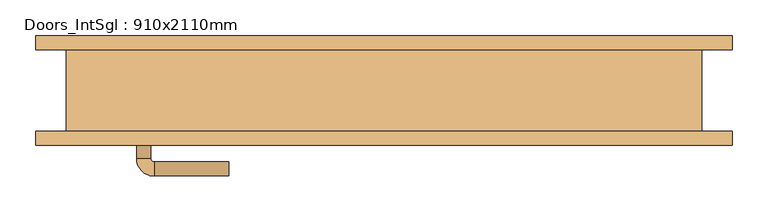
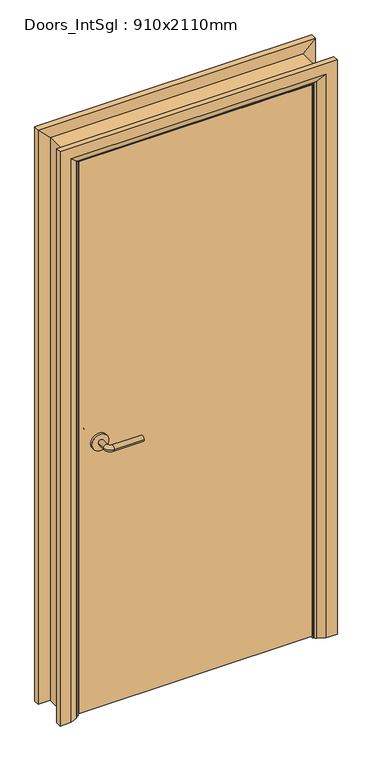
"""IFC4 building model written with IfcOpenShell, lengths in millimetres: door geometry, Doors_IntSgl : 910x2110mm."""

from ifc_helpers import new_model, si_unit, point, frame, frame_2d, origin, place, context, project, spatial, polyline, circle_curve, ellipse_curve, trimmed, segment, composite_curve, outline, extrude, faceted_brep, source, transform, mapped, element, save
from ifc_brep_helpers import plane_surface, cylinder_surface, revolved_surface, advanced_brep


def doors_intsgl_910x2110mm_8ca64813(model_context):
    return source(origin(), model_context, "Body", "SolidModel", [
        advanced_brep(
        [(-348.0, -11.15, 1000.0), (-328.0, -11.15, 1000.0), (-348.0, 18.85, 1000.0), (-328.0, 18.85, 1000.0), (-323.0, 23.85, 1000.0), (-323.0, 43.85, 1000.0), (-218.0, 43.85, 1000.0), (-218.0, 23.85, 1000.0)],
        [
            (0, 1, circle_curve(frame((-338.0, -11.15, 1000.0), z_axis=(0.0, -1.0, 0.0), x_axis=(1.0, 0.0, 0.0)), 10.0)),
            (1, 0, circle_curve(frame((-338.0, -11.15, 1000.0), z_axis=(0.0, -1.0, 0.0), x_axis=(1.0, 0.0, 0.0)), 10.0)),
            (0, 2),
            (2, 3, circle_curve(frame((-338.0, 18.85, 1000.0), z_axis=(0.0, -1.0, 0.0), x_axis=(1.0, 0.0, 0.0)), 10.0)),
            (3, 1),
            (3, 2, circle_curve(frame((-338.0, 18.85, 1000.0), z_axis=(0.0, -1.0, 0.0), x_axis=(1.0, 0.0, 0.0)), 10.0)),
            (4, 3, circle_curve(frame((-323.0, 18.85, 1000.0), z_axis=(0.0, 0.0, 1.0), x_axis=(-1.0, 0.0, 0.0)), 5.0)),
            (2, 5, circle_curve(frame((-323.0, 18.85, 1000.0), z_axis=(0.0, 0.0, -1.0), x_axis=(-1.0, 0.0, 0.0)), 25.0)),
            (5, 4, circle_curve(frame((-323.0, 33.85, 1000.0), z_axis=(-1.0, 0.0, 0.0), x_axis=(0.0, -1.0, 0.0)), 10.0)),
            (4, 5, circle_curve(frame((-323.0, 33.85, 1000.0), z_axis=(-1.0, 0.0, 0.0), x_axis=(0.0, -1.0, 0.0)), 10.0)),
            (6, 7, circle_curve(frame((-218.0, 33.85, 1000.0), z_axis=(1.0, 0.0, 0.0), x_axis=(0.0, -1.0, 0.0)), 10.0)),
            (7, 6, circle_curve(frame((-218.0, 33.85, 1000.0), z_axis=(1.0, 0.0, 0.0), x_axis=(0.0, -1.0, 0.0)), 10.0)),
            (5, 6),
            (7, 4),
        ],
        [
            plane_surface(frame((-338.0, -11.15, 1000.0), z_axis=(0.0, -1.0, 0.0), x_axis=(0.0, 0.0, 1.0))),
            cylinder_surface(frame((-338.0, -11.15, 1000.0), z_axis=(0.0, -1.0, 0.0), x_axis=(1.0, 0.0, 0.0)), 10.0),
            revolved_surface(trimmed(ellipse_curve(frame((-338.0, 18.85, 1000.0), z_axis=(0.0, -1.0, 0.0), x_axis=(1.0, 0.0, 0.0)), 10.0, 10.0), [point((-348.0, 18.85, 1000.0))], [point((-328.0, 18.85, 1000.0))], True, "CARTESIAN"), (-323.0, 18.85, 1000.0), (0.0, 0.0, -1.0)),
            revolved_surface(trimmed(ellipse_curve(frame((-338.0, 18.85, 1000.0), z_axis=(0.0, -1.0, 0.0), x_axis=(1.0, 0.0, 0.0)), 10.0, 10.0), [point((-328.0, 18.85, 1000.0))], [point((-348.0, 18.85, 1000.0))], True, "CARTESIAN"), (-323.0, 18.85, 1000.0), (0.0, 0.0, -1.0)),
            plane_surface(frame((-218.0, 33.85, 1000.0), z_axis=(1.0, 0.0, 0.0), x_axis=(0.0, 0.0, 1.0))),
            cylinder_surface(frame((-323.0, 33.85, 1000.0), z_axis=(-1.0, 0.0, 0.0), x_axis=(0.0, -1.0, 0.0)), 10.0),
        ],
        [
            (0, [[1, 2]]),
            (1, [[-1, 3, 4, 5]]),
            (1, [[-2, -5, 6, -3]]),
            (2, [[7, -4, 8, 9]]),
            (3, [[-8, -6, -7, 10]]),
            (4, [[11, 12]]),
            (5, [[-9, 13, -12, 14]]),
            (5, [[-10, -14, -11, -13]]),
        ],
    ),
        extrude(outline(composite_curve([segment(trimmed(circle_curve(frame_2d((1000.0, -340.5)), 30.0), [point((1000.0, -370.5))], [point((1000.0, -310.5))], False, "CARTESIAN"), True, "CONTINUOUS"), segment(trimmed(circle_curve(frame_2d((1000.0, -340.5)), 30.0), [point((1000.0, -310.5))], [point((1000.0, -370.5))], False, "CARTESIAN"), True, "CONTINUOUS")], self_intersect=False)), frame((0.0, -19.15, 0.0), z_axis=(0.0, 1.0, 0.0), x_axis=(0.0, 0.0, 1.0)), (0.0, 0.0, 1.0), 8.0),
        advanced_brep(
        [(-348.0, -65.15, 1000.0), (-328.0, -65.15, 1000.0), (-328.0, -95.15, 1000.0), (-348.0, -95.15, 1000.0), (-323.0, -100.15, 1000.0), (-323.0, -120.15, 1000.0), (-218.0, -120.15, 1000.0), (-218.0, -100.15, 1000.0)],
        [
            (0, 1, circle_curve(frame((-338.0, -65.15, 1000.0), z_axis=(0.0, 1.0, 0.0), x_axis=(1.0, 0.0, 0.0)), 10.0)),
            (1, 0, circle_curve(frame((-338.0, -65.15, 1000.0), z_axis=(0.0, 1.0, 0.0), x_axis=(1.0, 0.0, 0.0)), 10.0)),
            (1, 2),
            (2, 3, circle_curve(frame((-338.0, -95.15, 1000.0), z_axis=(0.0, 1.0, 0.0), x_axis=(1.0, 0.0, 0.0)), 10.0)),
            (3, 0),
            (3, 2, circle_curve(frame((-338.0, -95.15, 1000.0), z_axis=(0.0, 1.0, 0.0), x_axis=(1.0, 0.0, 0.0)), 10.0)),
            (4, 5, circle_curve(frame((-323.0, -110.15, 1000.0), z_axis=(-1.0, 0.0, 0.0), x_axis=(0.0, 1.0, 0.0)), 10.0)),
            (5, 3, circle_curve(frame((-323.0, -95.15, 1000.0), z_axis=(0.0, 0.0, -1.0), x_axis=(-1.0, 0.0, 0.0)), 25.0)),
            (2, 4, circle_curve(frame((-323.0, -95.15, 1000.0), z_axis=(0.0, 0.0, 1.0), x_axis=(-1.0, 0.0, 0.0)), 5.0)),
            (5, 4, circle_curve(frame((-323.0, -110.15, 1000.0), z_axis=(-1.0, 0.0, 0.0), x_axis=(0.0, 1.0, 0.0)), 10.0)),
            (6, 7, circle_curve(frame((-218.0, -110.15, 1000.0), z_axis=(1.0, 0.0, 0.0), x_axis=(0.0, 1.0, 0.0)), 10.0)),
            (7, 6, circle_curve(frame((-218.0, -110.15, 1000.0), z_axis=(1.0, 0.0, 0.0), x_axis=(0.0, 1.0, 0.0)), 10.0)),
            (4, 7),
            (6, 5),
        ],
        [
            plane_surface(frame((-338.0, -65.15, 1000.0), z_axis=(0.0, 1.0, 0.0), x_axis=(0.0, 0.0, 1.0))),
            cylinder_surface(frame((-338.0, -65.15, 1000.0), z_axis=(0.0, 1.0, 0.0), x_axis=(1.0, 0.0, 0.0)), 10.0),
            revolved_surface(trimmed(ellipse_curve(frame((-338.0, -95.15, 1000.0), z_axis=(0.0, -1.0, 0.0), x_axis=(1.0, 0.0, 0.0)), 10.0, 10.0), [point((-348.0, -95.15, 1000.0))], [point((-328.0, -95.15, 1000.0))], True, "CARTESIAN"), (-323.0, -95.15, 1000.0), (0.0, 0.0, -1.0)),
            revolved_surface(trimmed(ellipse_curve(frame((-338.0, -95.15, 1000.0), z_axis=(0.0, -1.0, 0.0), x_axis=(1.0, 0.0, 0.0)), 10.0, 10.0), [point((-328.0, -95.15, 1000.0))], [point((-348.0, -95.15, 1000.0))], True, "CARTESIAN"), (-323.0, -95.15, 1000.0), (0.0, 0.0, -1.0)),
            plane_surface(frame((-218.0, -110.15, 1000.0), z_axis=(1.0, 0.0, 0.0), x_axis=(0.0, 0.0, 1.0))),
            cylinder_surface(frame((-323.0, -110.15, 1000.0), z_axis=(-1.0, 0.0, 0.0), x_axis=(0.0, 1.0, 0.0)), 10.0),
        ],
        [
            (0, [[1, 2]]),
            (1, [[3, 4, 5, -2]]),
            (1, [[-5, 6, -3, -1]]),
            (2, [[7, 8, -4, 9]]),
            (3, [[10, -9, -6, -8]]),
            (4, [[11, 12]]),
            (5, [[13, -11, 14, -7]]),
            (5, [[-14, -12, -13, -10]]),
        ],
    ),
        extrude(outline(composite_curve([segment(trimmed(circle_curve(frame_2d((1000.0, -340.5)), 30.0), [point((1000.0, -370.5))], [point((1000.0, -310.5))], False, "CARTESIAN"), True, "CONTINUOUS"), segment(trimmed(circle_curve(frame_2d((1000.0, -340.5)), 30.0), [point((1000.0, -310.5))], [point((1000.0, -370.5))], False, "CARTESIAN"), True, "CONTINUOUS")], self_intersect=False)), frame((0.0, -65.15, 0.0), z_axis=(0.0, 1.0, 0.0), x_axis=(0.0, 0.0, 1.0)), (0.0, 0.0, 1.0), 8.0),
        extrude(outline(polyline([(413.0, -19.15), (413.0, -57.15), (-413.0, -57.15), (-413.0, -19.15), (413.0, -19.15)])), frame((0.0, 0.0, 8.0), z_axis=(0.0, 0.0, 1.0), x_axis=(1.0, 0.0, 0.0)), (0.0, 0.0, 1.0), 2060.0),
        advanced_brep(
        [(490.0, -77.15, 0.0), (450.0, -77.15, 0.0), (424.0, -63.15, 0.0), (420.0, -57.15, 0.0), (490.0, -57.15, 0.0), (490.0, -57.15, 2145.0), (490.0, -77.15, 2145.0), (420.0, -57.15, 2075.0), (-420.0, -57.15, 2075.0), (-420.0, -57.15, 0.0), (-490.0, -57.15, 0.0), (-490.0, -57.15, 2145.0), (424.0, -63.15, 2079.0), (450.0, -77.15, 2105.0), (-490.0, -77.15, 2145.0), (-490.0, -77.15, 0.0), (-450.0, -77.15, 0.0), (-450.0, -77.15, 2105.0), (-424.0, -63.15, 2079.0), (-424.0, -63.15, 0.0)],
        [
            (0, 1),
            (1, 2),
            (2, 3, circle_curve(frame((428.0, -56.15, 0.0), z_axis=(0.0, 0.0, -1.0), x_axis=(1.0, 0.0, 0.0)), 8.0622577)),
            (3, 4),
            (4, 0),
            (4, 5),
            (5, 6),
            (6, 0),
            (3, 7),
            (7, 8),
            (8, 9),
            (9, 10),
            (10, 11),
            (11, 5),
            (2, 12),
            (12, 7, ellipse_curve(frame((428.0, -56.15, 2083.0), z_axis=(0.7071067811865475, 0.0, -0.7071067811865475), x_axis=(-0.7071067811865474, 0.0, -0.7071067811865476)), 11.4017543, 8.0622577)),
            (1, 13),
            (13, 12),
            (6, 14),
            (14, 15),
            (15, 16),
            (16, 17),
            (17, 13),
            (11, 14),
            (12, 18),
            (18, 8, ellipse_curve(frame((-428.0, -56.15, 2083.0), z_axis=(0.7071067811865475, 0.0, 0.7071067811865475), x_axis=(0.7071067811865476, 0.0, -0.7071067811865474)), 11.4017543, 8.0622577)),
            (17, 18),
            (15, 10),
            (9, 19, circle_curve(frame((-428.0, -56.15, 0.0), z_axis=(0.0, 0.0, -1.0), x_axis=(-1.0, 0.0, 0.0)), 8.0622577)),
            (19, 16),
            (18, 19),
        ],
        [
            plane_surface(frame((420.0, -57.15, 0.0), z_axis=(0.0, 0.0, -1.0), x_axis=(0.0, 1.0, 0.0))),
            plane_surface(frame((490.0, -77.15, 0.0), z_axis=(1.0, 0.0, 0.0), x_axis=(0.0, 0.0, 1.0))),
            plane_surface(frame((490.0, -57.15, 0.0), z_axis=(0.0, 1.0, 0.0), x_axis=(0.0, 0.0, 1.0))),
            cylinder_surface(frame((428.0, -56.15, 0.0), z_axis=(0.0, 0.0, -1.0), x_axis=(1.0, 0.0, 0.0)), 8.0622577),
            plane_surface(frame((424.0, -63.15, 0.0), z_axis=(-0.4740998230350126, -0.880471099922178, 0.0), x_axis=(0.0, 0.0, 1.0))),
            plane_surface(frame((450.0, -77.15, 0.0), z_axis=(0.0, -1.0, 0.0), x_axis=(0.0, 0.0, 1.0))),
            plane_surface(frame((490.0, -77.15, 2145.0), z_axis=(0.0, 0.0, 1.0), x_axis=(-1.0, 0.0, 0.0))),
            cylinder_surface(frame((420.0, -56.15, 2083.0), z_axis=(1.0, 0.0, 0.0), x_axis=(0.0, 0.0, 1.0)), 8.0622577),
            plane_surface(frame((424.0, -63.15, 2079.0), z_axis=(0.0, -0.8804710999221764, -0.4740998230350154), x_axis=(-1.0, 0.0, 0.0))),
            plane_surface(frame((-420.0, -57.15, 0.0), z_axis=(0.0, 0.0, -1.0), x_axis=(0.0, 1.0, 0.0))),
            plane_surface(frame((-490.0, -77.15, 2145.0), z_axis=(-1.0, 0.0, 0.0), x_axis=(0.0, 0.0, -1.0))),
            cylinder_surface(frame((-428.0, -56.15, 2075.0), z_axis=(0.0, 0.0, 1.0), x_axis=(-1.0, 0.0, 0.0)), 8.0622577),
            plane_surface(frame((-424.0, -63.15, 2079.0), z_axis=(0.47409982303501824, -0.8804710999221749, 0.0), x_axis=(0.0, 0.0, -1.0))),
        ],
        [
            (0, [[1, 2, 3, 4, 5]]),
            (1, [[6, 7, 8, -5]]),
            (2, [[9, 10, 11, 12, 13, 14, -6, -4]]),
            (3, [[15, 16, -9, -3]]),
            (4, [[17, 18, -15, -2]]),
            (5, [[-8, 19, 20, 21, 22, 23, -17, -1]]),
            (6, [[-14, 24, -19, -7]]),
            (7, [[25, 26, -10, -16]]),
            (8, [[-23, 27, -25, -18]]),
            (9, [[28, -12, 29, 30, -21]]),
            (10, [[-13, -28, -20, -24]]),
            (11, [[31, -29, -11, -26]]),
            (12, [[-22, -30, -31, -27]]),
        ],
    ),
        extrude(outline(polyline([(0.0, -396.0), (2051.0, -396.0), (2051.0, 396.0), (0.0, 396.0), (0.0, 415.0), (2070.0, 415.0), (2070.0, -415.0), (0.0, -415.0), (0.0, -396.0)])), frame((0.0, -17.15, 0.0), z_axis=(0.0, 1.0, 0.0), x_axis=(0.0, 0.0, 1.0)), (0.0, 0.0, 1.0), 32.0),
        advanced_brep(
        [(-490.0, 77.15, 0.0), (-450.0, 77.15, 0.0), (-424.0, 63.15, 0.0), (-420.0, 57.15, 0.0), (-490.0, 57.15, 0.0), (-490.0, 57.15, 2145.0), (-490.0, 77.15, 2145.0), (-420.0, 57.15, 2075.0), (-424.0, 63.15, 2079.0), (-450.0, 77.15, 2105.0), (490.0, 57.15, 2145.0), (490.0, 77.15, 2145.0), (420.0, 57.15, 2075.0), (424.0, 63.15, 2079.0), (450.0, 77.15, 2105.0), (490.0, 77.15, 0.0), (490.0, 57.15, 0.0), (420.0, 57.15, 0.0), (424.0, 63.15, 0.0), (450.0, 77.15, 0.0)],
        [
            (0, 1),
            (1, 2),
            (2, 3, circle_curve(frame((-428.0, 56.15, 0.0), z_axis=(0.0, 0.0, -1.0), x_axis=(-1.0, 0.0, 0.0)), 8.0622577)),
            (3, 4),
            (4, 0),
            (4, 5),
            (5, 6),
            (6, 0),
            (3, 7),
            (7, 5),
            (2, 8),
            (8, 7, ellipse_curve(frame((-428.0, 56.15, 2083.0), z_axis=(-0.7071067811865475, 0.0, -0.7071067811865475), x_axis=(0.7071067811865474, 0.0, -0.7071067811865476)), 11.4017543, 8.0622577)),
            (1, 9),
            (9, 8),
            (6, 9),
            (5, 10),
            (10, 11),
            (11, 6),
            (7, 12),
            (12, 10),
            (8, 13),
            (13, 12, ellipse_curve(frame((428.0, 56.15, 2083.0), z_axis=(-0.7071067811865475, 0.0, 0.7071067811865475), x_axis=(-0.7071067811865476, 0.0, -0.7071067811865474)), 11.4017543, 8.0622577)),
            (9, 14),
            (14, 13),
            (11, 14),
            (15, 16),
            (16, 17),
            (17, 18, circle_curve(frame((428.0, 56.15, 0.0), z_axis=(0.0, 0.0, -1.0), x_axis=(1.0, 0.0, 0.0)), 8.0622577)),
            (18, 19),
            (19, 15),
            (10, 16),
            (15, 11),
            (12, 17),
            (13, 18),
            (14, 19),
        ],
        [
            plane_surface(frame((-420.0, 129.9510989, 0.0), z_axis=(0.0, 0.0, -1.0), x_axis=(1.0, 0.0, 0.0))),
            plane_surface(frame((-490.0, 77.15, 0.0), z_axis=(-1.0, 0.0, 0.0), x_axis=(0.0, 0.0, 1.0))),
            plane_surface(frame((-490.0, 57.15, 0.0), z_axis=(0.0, -1.0, 0.0), x_axis=(0.0, 0.0, 1.0))),
            cylinder_surface(frame((-428.0, 56.15, 0.0), z_axis=(0.0, 0.0, -1.0), x_axis=(-1.0, 0.0, 0.0)), 8.0622577),
            plane_surface(frame((-424.0, 63.15, 0.0), z_axis=(0.4740998230350183, 0.8804710999221749, 0.0), x_axis=(0.0, 0.0, 1.0))),
            plane_surface(frame((-450.0, 77.15, 0.0), z_axis=(0.0, 1.0, 0.0), x_axis=(0.0, 0.0, 1.0))),
            plane_surface(frame((-490.0, 77.15, 2145.0), z_axis=(0.0, 0.0, 1.0), x_axis=(1.0, 0.0, 0.0))),
            plane_surface(frame((-490.0, 57.15, 2145.0), z_axis=(0.0, -1.0, 0.0), x_axis=(1.0, 0.0, 0.0))),
            cylinder_surface(frame((-420.0, 56.15, 2083.0), z_axis=(-1.0, 0.0, 0.0), x_axis=(0.0, 0.0, 1.0)), 8.0622577),
            plane_surface(frame((-424.0, 63.15, 2079.0), z_axis=(0.0, 0.8804710999221749, -0.4740998230350183), x_axis=(1.0, 0.0, 0.0))),
            plane_surface(frame((-450.0, 77.15, 2105.0), z_axis=(0.0, 1.0, 0.0), x_axis=(1.0, 0.0, 0.0))),
            plane_surface(frame((420.0, 129.9510989, 0.0), z_axis=(0.0, 0.0, -1.0), x_axis=(-1.0, 0.0, 0.0))),
            plane_surface(frame((490.0, 77.15, 2145.0), z_axis=(1.0, 0.0, 0.0), x_axis=(0.0, 0.0, -1.0))),
            plane_surface(frame((490.0, 57.15, 2145.0), z_axis=(0.0, -1.0, 0.0), x_axis=(0.0, 0.0, -1.0))),
            cylinder_surface(frame((428.0, 56.15, 2075.0), z_axis=(0.0, 0.0, 1.0), x_axis=(1.0, 0.0, 0.0)), 8.0622577),
            plane_surface(frame((424.0, 63.15, 2079.0), z_axis=(-0.4740998230350183, 0.8804710999221749, 0.0), x_axis=(0.0, 0.0, -1.0))),
            plane_surface(frame((450.0, 77.15, 2105.0), z_axis=(0.0, 1.0, 0.0), x_axis=(0.0, 0.0, -1.0))),
        ],
        [
            (0, [[1, 2, 3, 4, 5]]),
            (1, [[6, 7, 8, -5]]),
            (2, [[9, 10, -6, -4]]),
            (3, [[11, 12, -9, -3]]),
            (4, [[13, 14, -11, -2]]),
            (5, [[-8, 15, -13, -1]]),
            (6, [[16, 17, 18, -7]]),
            (7, [[19, 20, -16, -10]]),
            (8, [[21, 22, -19, -12]]),
            (9, [[23, 24, -21, -14]]),
            (10, [[-18, 25, -23, -15]]),
            (11, [[26, 27, 28, 29, 30]]),
            (12, [[31, -26, 32, -17]]),
            (13, [[33, -27, -31, -20]]),
            (14, [[34, -28, -33, -22]]),
            (15, [[35, -29, -34, -24]]),
            (16, [[-32, -30, -35, -25]]),
        ],
    ),
        faceted_brep([(-415.0, -57.15, 0.0), (-447.0, -57.15, 0.0), (-447.0, 57.15, 0.0), (-415.0, 57.15, 0.0), (-415.0, 57.15, 2070.0), (-415.0, -57.15, 2070.0), (-447.0, 57.15, 2102.0), (-447.0, -57.15, 2102.0), (415.0, 57.15, 2070.0), (415.0, -57.15, 2070.0), (447.0, 57.15, 2102.0), (447.0, -57.15, 2102.0), (415.0, -57.15, 0.0), (415.0, 57.15, 0.0), (447.0, 57.15, 0.0), (447.0, -57.15, 0.0)], [[[0, 1, 2, 3]], [[3, 4, 5, 0]], [[2, 6, 4, 3]], [[1, 7, 6, 2]], [[0, 5, 7, 1]], [[4, 8, 9, 5]], [[6, 10, 8, 4]], [[7, 11, 10, 6]], [[5, 9, 11, 7]], [[12, 13, 14, 15]], [[8, 13, 12, 9]], [[10, 14, 13, 8]], [[11, 15, 14, 10]], [[9, 12, 15, 11]]]),
    ])


if __name__ == "__main__":
    model = new_model("IFC4")
    model_context = context("Model", 3, world=origin())
    ifc_project = project(units=[si_unit("LENGTHUNIT", "METRE", prefix="MILLI")], contexts=[model_context])
    site = spatial("IfcSite", under=ifc_project)
    building = spatial("IfcBuilding", under=site)
    placement = place(None, origin())
    doors_intsgl_910x2110mm_shape = doors_intsgl_910x2110mm_8ca64813(model_context)
    element("IfcDoor", 1, ObjectType="Doors_IntSgl : 910x2110mm", at=placement, inside=building, context=model_context, shape_type="MappedRepresentation", body=[
        mapped(doors_intsgl_910x2110mm_shape, transform((0.0, 0.0, 0.0), x_axis=(1.0, 0.0, 0.0), y_axis=(0.0, 1.0, 0.0), z_axis=(0.0, 0.0, 1.0))),
    ])
    save(model, "model.ifc")

# Revit data of these elements
# Type "Doors_IntSgl : 910x2110mm"
#   Construction Type Id = "MDOOR"
#   Type Mark = "41"
#   Type Comments = "Internal Single"
#   Operation = "SingleSwingRight"
#   Manufacturer = "Revit"
#   Keynote = "L20"
#   Description = "Internal Single Door"
#   Analytic Construction = "Metal"
#   UnderCut = 0' - 0.31496"
#   Tolerance = 0' - 0.07874"
#   Thickness = 0' - 1.49606"
#   Thermal Resistance (R) = 0.270117 (m²·K)/W
#   Structural Tolerance = 0' - 0.31496"
#   StopDepth = 0' - 1.25984"
#   Stop Thickness = 0' - 0.74803"
#   Rough Width = 2' - 11.82677"
#   Rough Height = 6' - 11.07087"
#   Height to Top Lock Rail = 3' - 3.37008"
#   Heat Transfer Coefficient (U) = 3.7021 W/(m²·K)
#   Handle Z Distance = 3' - 3.37008"
#   Handle X Distance = 0' - 2.95276"
#   Frame Thickness = 0' - 1.25984"
#   Door Panel Width = 2' - 8.51969"
#   Door Panel Thickness = 0' - 1.49606"
#   Door Panel Offset = 0' - 0"
#   Height = 6' - 11.07087"
#   Width = 2' - 11.82677"
#   Door Panel Height = 6' - 9.10236"
#   Architrave Setback = 0' - 0.19685"
#   Define Thermal Properties by = 1
#   Vis - Ironmongery = yes
#   Material Ironmongery = Door - Handle
#   Material Frame = Door - Frame/Mullion (1)
#   Material Door = Door - Panel
#   Material Architrave = Door - Architrave
#   Visual Light Transmittance = 0
#   Solar Heat Gain Coefficient = 0
#   Function = (empty or 0)
#   Wall Closure = (empty or 0)
# Element 1 (IfcDoor, "Doors_IntSgl : 910x2110mm")
#   Materials on its faces: "Door - Architrave", "Door - Handle", "Door - Frame/Mullion (1)", "Door - Panel"
# Materials
#   "Door - Handle": colour RGB 17 17 17, transparency 0, Keynote = "P21", Cost = 0
#   "Door - Frame/Mullion (1)": class "Wood", colour RGB 212 179 113, transparency 0, Keynote = "L20", Cost = 0
#   "Door - Panel": class "Wood", colour RGB 210 159 95, transparency 0, Keynote = "L20", Cost = 0
#   "Door - Architrave": class "Wood", colour RGB 154 90 5, transparency 0, Keynote = "P20", Cost = 0
